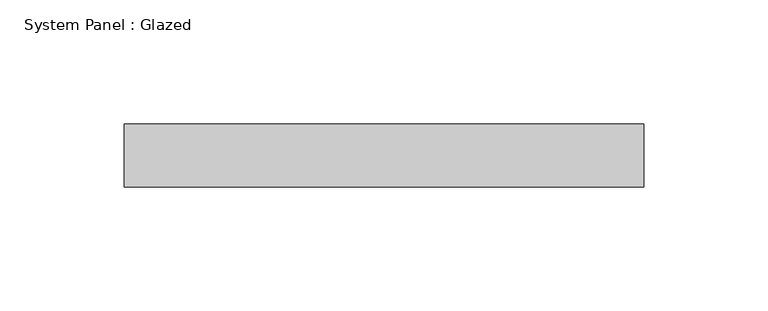
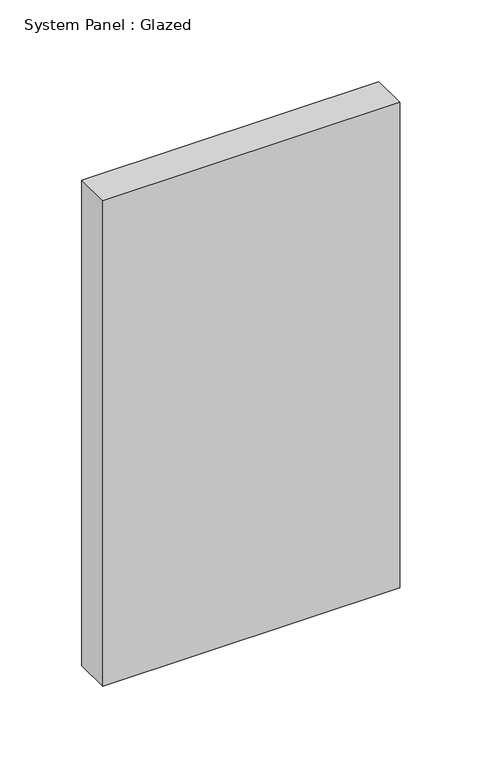
"""IFC4 building model written with IfcOpenShell, lengths in millimetres: plate geometry, System Panel : Glazed."""

from ifc_helpers import new_model, si_unit, origin, origin_with_axes, place, context, project, spatial, polyline, outline, extrude, source, transform, mapped, element, save


def system_panel_glazed_94a389e0(model_context):
    return source(origin(), model_context, "Body", "SweptSolid", [
        extrude(outline(polyline([(104.775, 19.05), (-104.775, 19.05), (-104.775, 44.45), (104.775, 44.45), (104.775, 19.05)])), origin_with_axes(), (0.0, 0.0, 1.0), 361.95),
    ])


if __name__ == "__main__":
    model = new_model("IFC4")
    model_context = context("Model", 3, world=origin())
    ifc_project = project(units=[si_unit("LENGTHUNIT", "METRE", prefix="MILLI")], contexts=[model_context])
    site = spatial("IfcSite", under=ifc_project)
    building = spatial("IfcBuilding", under=site)
    placement = place(None, origin())
    system_panel_glazed_shape = system_panel_glazed_94a389e0(model_context)
    element("IfcPlate", 1, ObjectType="System Panel : Glazed", at=placement, inside=building, context=model_context, shape_type="MappedRepresentation", body=[
        mapped(system_panel_glazed_shape, transform((0.0, 0.0, 0.0), x_axis=(1.0, 0.0, 0.0), y_axis=(0.0, 1.0, 0.0), z_axis=(0.0, 0.0, 1.0))),
    ])
    save(model, "model.ifc")

# Revit data of these elements
# Type "System Panel : Glazed"
#   Construction Type Id = "GSP4R"
#   Analytic Construction = "1/8 in Pilkington single glazing"
#   Visual Light Transmittance = 0.9
#   Solar Heat Gain Coefficient = 0.86
#   Heat Transfer Coefficient (U) = 1.18115 BTU/(h·ft²·°F)
#   Define Thermal Properties by = 1
# Element 1 (IfcPlate, "System Panel : Glazed")
#   Materials on its faces: "Glass"
# Materials
#   "Glass": class "Glass", colour RGB 0 128 192, transparency 0.75, Description = "Soda Lime Glass", Cost = 0
